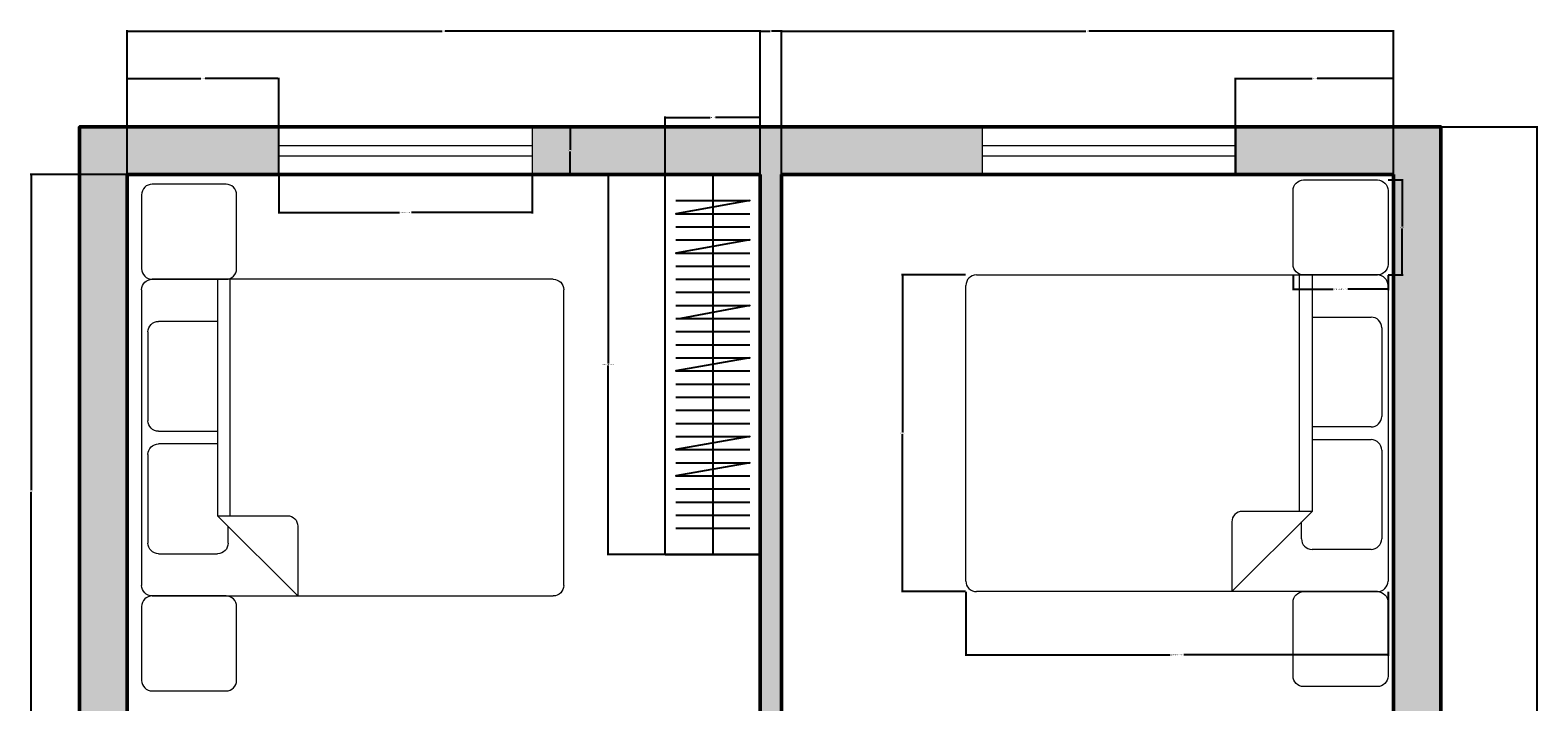
# Model space of a CAD drawing. Units: inches. Extents: x 2130 to 2425, y 2862 to 3216.
# Tile 4 of 4: x 2139 to 2425, y 3089 to 3216. Entities that reach past the tile are written whole.
import ezdxf

# ---------------------------------------------------------------- set-up
doc = ezdxf.new("R2010")
doc.units = ezdxf.units.IN
for name, color, linetype, lineweight in [('A-ANNO-DIMS', 2, 'Continuous', 18), ('A-FLOR-CASE', 9, 'Continuous', 25), ('A-FURN', 8, 'Continuous', 18), ('A-GLAZ', 4, 'Continuous', 18), ('A-WALL', 7, 'Continuous', 50), ('A-WALL-PATT', 18, 'Continuous', 13)]:
    doc.layers.add(name, color=color, linetype=linetype, lineweight=lineweight)
doc.styles.get("Standard").update_dxf_attribs({"font": 'arial.ttf'})
doc.dimstyles.get("Standard").update_dxf_attribs({"dimtxt": 0.18, "dimasz": 0.18, "dimexe": 0.18, "dimexo": 0.0625, "dimgap": 0.09, "dimtad": 0, "dimtih": 1, "dimtoh": 1, "dimdec": 4, "dimzin": 0, "dimdsep": 46, "dimtxsty": 'Standard', "dimcen": 0.09, "dimadec": 0, "dimazin": 0, "dimtfac": 1, "dimtdec": 4, "dimtofl": 0, "dimtmove": 0, "dimatfit": 3, "dimfxl": 1, "dimtolj": 1, "dimtzin": 0, "dimarcsym": 0})

# ---------------------------------------------------------------- blocks, each defined once
blk = doc.blocks.new('Bed - Queen')
for p, q in [((2, 0), (57.99999, 0)), ((0, -78.00003), (0, -2)), ((9.99999, -1.2), (26.79998, -1.2)), ((33.19999, -1.2), (49.99999, -1.2)), ((59.99999, -2), (59.99999, -78.00003)), ((7.99999, -14.4), (7.99999, -3.2)), ((28.79998, -3.2), (28.79998, -14.4)), ((31.19999, -14.4), (31.19999, -3.2)), ((51.99999, -3.2), (51.99999, -14.4)), ((0, -14.4), (44.8, -14.4)), ((44.8, -16.8), (0, -16.8)), ((59.99999, -29.6), (44.8, -14.4)), ((44.8, -14.4), (44.8, -27.6)), ((49.99999, -16.4), (46.79936, -16.4)), ((46.8, -29.6), (59.99999, -29.6)), ((57.99999, -80.00003), (2, -80.00003))]:
    blk.add_line(p, q)
for centre, start, end in [((2, -2), 90, 180), ((57.99999, -2), 0, 90), ((9.99999, -3.2), 90, 180), ((26.79998, -3.2), 0, 90), ((33.19999, -3.2), 90, 180), ((49.99999, -3.2), 0, 90), ((49.99999, -14.4), 270, 0), ((46.8, -27.6), 180, 270), ((2, -78.00003), 180, 270), ((57.99999, -78.00003), 270, 0)]:
    blk.add_arc(centre, 2, start, end)
blk = doc.blocks.new('WIN-48IN')
for p, q in [((0, 0), (0, 9)), ((48, 9), (48, 0)), ((0, 5.5), (48, 5.5)), ((0, 3.5), (48, 3.5))]:
    blk.add_line(p, q)
blk = doc.blocks.new('WARDROBE-72X18IN')
for p, q in [((0, 0), (0, 72)), ((0, 72), (18, 72)), ((9, 72), (9, 0)), ((18, 72), (18, 0)), ((2, 62.07), (16, 62.07)), ((2, 54.62), (16, 54.62)), ((2, 52.14), (16, 52.14)), ((2, 49.66), (16, 49.66)), ((2, 44.69), (16, 44.69)), ((2, 42.21), (16, 42.21)), ((2, 39.72), (16, 39.72)), ((2, 32.28), (16, 32.28)), ((2, 29.79), (16, 29.79)), ((2, 27.31), (16, 27.31)), ((2, 24.83), (16, 24.83)), ((2, 12.41), (16, 12.41)), ((2, 9.93), (16, 9.93)), ((2, 7.45), (16, 7.45)), ((2, 4.97), (16, 4.97)), ((18, 0), (0, 0))]:
    blk.add_line(p, q)
for points in [[(2, 67.03), (16, 67.03), (2, 64.55), (16, 64.55)], [(2, 59.59), (16, 59.59), (2, 57.1), (16, 57.1)], [(2, 47.17), (16, 47.17), (2.98, 44.69)], [(2, 37.24), (16, 37.24), (2, 34.76), (16, 34.76)], [(2, 22.35), (16, 22.35), (2, 19.86), (16, 19.86)], [(2, 17.38), (16, 17.38), (2, 14.9), (16, 14.9)]]:
    blk.add_lwpolyline(points)
blk.add_lwpolyline([(0, 0), (18, 0)], close=True)
blk = doc.blocks.new('NIGHTSTAND-18IN')
blk.add_lwpolyline([(16, 0), (2, 0, -0.414214), (0, 2), (0, 16, -0.414214), (2, 18), (16, 18, -0.414214), (18, 16), (18, 2, -0.414214)], format="xyb", close=True)
blk = doc.blocks.new('*D15')
at = {"layer": 'A-ANNO-DIMS', "color": 0, "lineweight": -2, "transparency": 16777216}
for p, q in [((2186.32, 3188.89), (2186.32, 3181.57)), ((2234.32, 3188.89), (2234.32, 3181.57)), ((2186.5, 3181.75), (2209.2, 3181.75)), ((2234.14, 3181.75), (2211.44, 3181.75))]:
    blk.add_line(p, q, dxfattribs=at)
at = {"layer": 'A-ANNO-DIMS', "color": 0, "transparency": 16777216}
for points in [[(2186.5, 3181.78), (2186.5, 3181.72), (2186.32, 3181.75)], [(2234.14, 3181.78), (2234.14, 3181.72), (2234.32, 3181.75)]]:
    blk.add_solid(points, dxfattribs=at)
at = {"layer": 'Defpoints', "color": 0, "transparency": 16777216}
for p in [(2186.32, 3188.95), (2234.32, 3188.95), (2234.32, 3181.75)]:
    blk.add_point(p, dxfattribs=at)
at = {"layer": 'A-ANNO-DIMS', "color": 0, "transparency": 16777216, "insert": (2210.32, 3181.75), "char_height": 0.18, "attachment_point": 5}
blk.add_mtext('\\A1;WINDOW 48 TYP.', dxfattribs=at)
blk = doc.blocks.new('*D16')
at = {"layer": 'A-ANNO-DIMS', "color": 0, "lineweight": -2, "transparency": 16777216}
for p, q in [((2234.39, 3197.95), (2241.7, 3197.95)), ((2241.52, 3197.77), (2241.52, 3193.64)), ((2241.52, 3189.13), (2241.52, 3193.27)), ((2234.39, 3188.95), (2241.7, 3188.95))]:
    blk.add_line(p, q, dxfattribs=at)
at = {"layer": 'A-ANNO-DIMS', "color": 0, "transparency": 16777216}
for points in [[(2241.49, 3197.77), (2241.55, 3197.77), (2241.52, 3197.95)], [(2241.49, 3189.13), (2241.55, 3189.13), (2241.52, 3188.95)]]:
    blk.add_solid(points, dxfattribs=at)
at = {"layer": 'Defpoints', "color": 0, "transparency": 16777216}
for p in [(2234.32, 3197.95), (2241.52, 3197.95), (2234.32, 3188.95)]:
    blk.add_point(p, dxfattribs=at)
at = {"layer": 'A-ANNO-DIMS', "color": 0, "transparency": 16777216, "insert": (2241.52, 3193.45), "char_height": 0.18, "attachment_point": 5}
blk.add_mtext('\\A1;9 TYP.', dxfattribs=at)
blk = doc.blocks.new('*D17')
at = {"layer": 'A-ANNO-DIMS', "color": 0, "lineweight": -2, "transparency": 16777216}
for p, q in [((2378.51, 3169.85), (2378.51, 3167.03)), ((2396.51, 3169.85), (2396.51, 3167.03)), ((2378.69, 3167.21), (2386.13, 3167.21)), ((2396.33, 3167.21), (2388.89, 3167.21))]:
    blk.add_line(p, q, dxfattribs=at)
at = {"layer": 'A-ANNO-DIMS', "color": 0, "transparency": 16777216}
for points in [[(2378.69, 3167.24), (2378.69, 3167.18), (2378.51, 3167.21)], [(2396.33, 3167.24), (2396.33, 3167.18), (2396.51, 3167.21)]]:
    blk.add_solid(points, dxfattribs=at)
at = {"layer": 'Defpoints', "color": 0, "transparency": 16777216}
for p in [(2378.51, 3169.91), (2396.51, 3169.91), (2396.51, 3167.21)]:
    blk.add_point(p, dxfattribs=at)
at = {"layer": 'A-ANNO-DIMS', "color": 0, "transparency": 16777216, "insert": (2387.51, 3167.21), "char_height": 0.18, "attachment_point": 5}
blk.add_mtext('\\A1;NIGHTSTAND 18 TYP.', dxfattribs=at)
blk = doc.blocks.new('*D18')
at = {"layer": 'A-ANNO-DIMS', "color": 0, "lineweight": -2, "transparency": 16777216}
for p, q in [((2396.57, 3187.91), (2399.39, 3187.91)), ((2399.21, 3187.73), (2399.21, 3179.09)), ((2399.21, 3170.09), (2399.21, 3178.73)), ((2396.57, 3169.91), (2399.39, 3169.91))]:
    blk.add_line(p, q, dxfattribs=at)
at = {"layer": 'A-ANNO-DIMS', "color": 0, "transparency": 16777216}
for points in [[(2399.18, 3187.73), (2399.24, 3187.73), (2399.21, 3187.91)], [(2399.18, 3170.09), (2399.24, 3170.09), (2399.21, 3169.91)]]:
    blk.add_solid(points, dxfattribs=at)
at = {"layer": 'Defpoints', "color": 0, "transparency": 16777216}
for p in [(2396.51, 3187.91), (2399.21, 3187.91), (2396.51, 3169.91)]:
    blk.add_point(p, dxfattribs=at)
at = {"layer": 'A-ANNO-DIMS', "color": 0, "transparency": 16777216, "insert": (2399.21, 3178.91), "char_height": 0.18, "attachment_point": 5}
blk.add_mtext('\\A1;18 TYP.', dxfattribs=at)
blk = doc.blocks.new('*D19')
at = {"layer": 'A-ANNO-DIMS', "color": 0, "lineweight": -2, "transparency": 16777216}
for p, q in [((2259.49, 3188.95), (2248.57, 3188.95)), ((2248.75, 3188.77), (2248.75, 3153.14)), ((2248.75, 3117.13), (2248.75, 3152.77)), ((2259.49, 3116.95), (2248.57, 3116.95))]:
    blk.add_line(p, q, dxfattribs=at)
at = {"layer": 'A-ANNO-DIMS', "color": 0, "transparency": 16777216}
for points in [[(2248.72, 3188.77), (2248.78, 3188.77), (2248.75, 3188.95)], [(2248.72, 3117.13), (2248.78, 3117.13), (2248.75, 3116.95)]]:
    blk.add_solid(points, dxfattribs=at)
at = {"layer": 'Defpoints', "color": 0, "transparency": 16777216}
for p in [(2248.75, 3188.95), (2259.55, 3188.95), (2259.55, 3116.95)]:
    blk.add_point(p, dxfattribs=at)
at = {"layer": 'A-ANNO-DIMS', "color": 0, "transparency": 16777216, "insert": (2248.75, 3152.95), "char_height": 0.18, "attachment_point": 5}
blk.add_mtext('\\A1;WARDROBE 72 TYP.', dxfattribs=at)
blk = doc.blocks.new('*D20')
at = {"layer": 'A-ANNO-DIMS', "color": 0, "lineweight": -2, "transparency": 16777216}
for p, q in [((2259.55, 3189.02), (2259.55, 3199.93)), ((2259.73, 3199.75), (2268.03, 3199.75)), ((2277.37, 3199.75), (2269.07, 3199.75)), ((2277.55, 3189.02), (2277.55, 3199.93))]:
    blk.add_line(p, q, dxfattribs=at)
at = {"layer": 'A-ANNO-DIMS', "color": 0, "transparency": 16777216}
for points in [[(2259.73, 3199.78), (2259.73, 3199.72), (2259.55, 3199.75)], [(2277.37, 3199.78), (2277.37, 3199.72), (2277.55, 3199.75)]]:
    blk.add_solid(points, dxfattribs=at)
at = {"layer": 'Defpoints', "color": 0, "transparency": 16777216}
for p in [(2277.55, 3199.75), (2259.55, 3188.95), (2277.55, 3188.95)]:
    blk.add_point(p, dxfattribs=at)
at = {"layer": 'A-ANNO-DIMS', "color": 0, "transparency": 16777216, "insert": (2268.55, 3199.75), "char_height": 0.18, "attachment_point": 5}
blk.add_mtext('\\A1;18 TYP.', dxfattribs=at)
blk = doc.blocks.new('*D27')
at = {"layer": 'A-ANNO-DIMS', "color": 0, "lineweight": -2, "transparency": 16777216}
for p, q in [((2316.51, 3109.85), (2316.51, 3097.73)), ((2396.51, 3109.85), (2396.51, 3097.73)), ((2316.69, 3097.91), (2355.21, 3097.91)), ((2396.33, 3097.91), (2357.81, 3097.91))]:
    blk.add_line(p, q, dxfattribs=at)
at = {"layer": 'A-ANNO-DIMS', "color": 0, "transparency": 16777216}
for points in [[(2316.69, 3097.94), (2316.69, 3097.88), (2316.51, 3097.91)], [(2396.33, 3097.94), (2396.33, 3097.88), (2396.51, 3097.91)]]:
    blk.add_solid(points, dxfattribs=at)
at = {"layer": 'Defpoints', "color": 0, "transparency": 16777216}
for p in [(2316.51, 3109.91), (2396.51, 3109.91), (2396.51, 3097.91)]:
    blk.add_point(p, dxfattribs=at)
at = {"layer": 'A-ANNO-DIMS', "color": 0, "transparency": 16777216, "insert": (2356.51, 3097.91), "char_height": 0.18, "attachment_point": 5}
blk.add_mtext('\\A1;QUEEN BED 80 TYP.', dxfattribs=at)
blk = doc.blocks.new('*D28')
at = {"layer": 'A-ANNO-DIMS', "color": 0, "lineweight": -2, "transparency": 16777216}
for p, q in [((2316.45, 3169.91), (2304.33, 3169.91)), ((2304.51, 3169.73), (2304.51, 3140.09)), ((2304.51, 3110.09), (2304.51, 3139.73)), ((2316.45, 3109.91), (2304.33, 3109.91))]:
    blk.add_line(p, q, dxfattribs=at)
at = {"layer": 'A-ANNO-DIMS', "color": 0, "transparency": 16777216}
for points in [[(2304.48, 3169.73), (2304.54, 3169.73), (2304.51, 3169.91)], [(2304.48, 3110.09), (2304.54, 3110.09), (2304.51, 3109.91)]]:
    blk.add_solid(points, dxfattribs=at)
at = {"layer": 'Defpoints', "color": 0, "transparency": 16777216}
for p in [(2316.51, 3169.91), (2304.51, 3109.91), (2316.51, 3109.91)]:
    blk.add_point(p, dxfattribs=at)
at = {"layer": 'A-ANNO-DIMS', "color": 0, "transparency": 16777216, "insert": (2304.51, 3139.91), "char_height": 0.18, "attachment_point": 5}
blk.add_mtext('\\A1;60 TYP.', dxfattribs=at)
blk = doc.blocks.new('*D36')
at = {"layer": 'A-ANNO-DIMS', "color": 0, "lineweight": -2, "transparency": 16777216}
for p, q in [((2406.61, 3197.95), (2424.88, 3197.95)), ((2424.7, 3197.77), (2424.7, 3039.14)), ((2424.7, 2880.13), (2424.7, 3038.77)), ((2406.61, 2879.95), (2424.88, 2879.95))]:
    blk.add_line(p, q, dxfattribs=at)
at = {"layer": 'A-ANNO-DIMS', "color": 0, "transparency": 16777216}
for points in [[(2424.67, 3197.77), (2424.73, 3197.77), (2424.7, 3197.95)], [(2424.67, 2880.13), (2424.73, 2880.13), (2424.7, 2879.95)]]:
    blk.add_solid(points, dxfattribs=at)
at = {"layer": 'Defpoints', "color": 0, "transparency": 16777216}
for p in [(2406.55, 3197.95), (2424.7, 3197.95), (2406.55, 2879.95)]:
    blk.add_point(p, dxfattribs=at)
at = {"layer": 'A-ANNO-DIMS', "color": 0, "transparency": 16777216, "insert": (2424.7, 3038.95), "char_height": 0.18, "attachment_point": 5}
blk.add_mtext('\\A1;318', dxfattribs=at)
blk = doc.blocks.new('*D37')
at = {"layer": 'A-ANNO-DIMS', "color": 0, "lineweight": -2, "transparency": 16777216}
for p, q in [((2157.55, 3189.02), (2157.55, 3207.28)), ((2157.73, 3207.1), (2171.54, 3207.1)), ((2186.14, 3207.1), (2172.33, 3207.1)), ((2186.32, 3189.02), (2186.32, 3207.28))]:
    blk.add_line(p, q, dxfattribs=at)
at = {"layer": 'A-ANNO-DIMS', "color": 0, "transparency": 16777216}
for points in [[(2157.73, 3207.13), (2157.73, 3207.07), (2157.55, 3207.1)], [(2186.14, 3207.13), (2186.14, 3207.07), (2186.32, 3207.1)]]:
    blk.add_solid(points, dxfattribs=at)
at = {"layer": 'Defpoints', "color": 0, "transparency": 16777216}
for p in [(2186.32, 3207.1), (2157.55, 3188.95), (2186.32, 3188.95)]:
    blk.add_point(p, dxfattribs=at)
at = {"layer": 'A-ANNO-DIMS', "color": 0, "transparency": 16777216, "insert": (2171.94, 3207.1), "char_height": 0.18, "attachment_point": 5}
blk.add_mtext('\\A1;28.77', dxfattribs=at)
blk = doc.blocks.new('*D38')
at = {"layer": 'A-ANNO-DIMS', "color": 0, "lineweight": -2, "transparency": 16777216}
for p, q in [((2367.64, 3189.02), (2367.64, 3207.28)), ((2367.82, 3207.1), (2382.13, 3207.1)), ((2397.37, 3207.1), (2383.06, 3207.1)), ((2397.55, 3189.02), (2397.55, 3207.28))]:
    blk.add_line(p, q, dxfattribs=at)
at = {"layer": 'A-ANNO-DIMS', "color": 0, "transparency": 16777216}
for points in [[(2367.82, 3207.13), (2367.82, 3207.07), (2367.64, 3207.1)], [(2397.37, 3207.13), (2397.37, 3207.07), (2397.55, 3207.1)]]:
    blk.add_solid(points, dxfattribs=at)
at = {"layer": 'Defpoints', "color": 0, "transparency": 16777216}
for p in [(2397.55, 3207.1), (2367.64, 3188.95), (2397.55, 3188.95)]:
    blk.add_point(p, dxfattribs=at)
at = {"layer": 'A-ANNO-DIMS', "color": 0, "transparency": 16777216, "insert": (2382.6, 3207.1), "char_height": 0.18, "attachment_point": 5}
blk.add_mtext('\\A1;29.907', dxfattribs=at)
blk = doc.blocks.new('*D46')
at = {"layer": 'A-ANNO-DIMS', "color": 0, "lineweight": -2, "transparency": 16777216}
for p, q in [((2157.55, 3189.02), (2157.55, 3216.28)), ((2157.73, 3216.1), (2217.27, 3216.1)), ((2277.37, 3216.1), (2217.83, 3216.1)), ((2277.55, 3189.02), (2277.55, 3216.28))]:
    blk.add_line(p, q, dxfattribs=at)
at = {"layer": 'A-ANNO-DIMS', "color": 0, "transparency": 16777216}
for points in [[(2157.73, 3216.13), (2157.73, 3216.07), (2157.55, 3216.1)], [(2277.37, 3216.13), (2277.37, 3216.07), (2277.55, 3216.1)]]:
    blk.add_solid(points, dxfattribs=at)
at = {"layer": 'Defpoints', "color": 0, "transparency": 16777216}
for p in [(2277.55, 3216.1), (2157.55, 3188.95), (2277.55, 3188.95)]:
    blk.add_point(p, dxfattribs=at)
at = {"layer": 'A-ANNO-DIMS', "color": 0, "transparency": 16777216, "insert": (2217.55, 3216.1), "char_height": 0.18, "attachment_point": 5}
blk.add_mtext('\\A1;120', dxfattribs=at)
blk = doc.blocks.new('*D47')
at = {"layer": 'A-ANNO-DIMS', "color": 0, "lineweight": -2, "transparency": 16777216}
for p, q in [((2277.55, 3189.02), (2277.55, 3216.28)), ((2277.73, 3216.1), (2279.4, 3216.1)), ((2281.37, 3216.1), (2279.7, 3216.1)), ((2281.55, 3189.02), (2281.55, 3216.28))]:
    blk.add_line(p, q, dxfattribs=at)
at = {"layer": 'A-ANNO-DIMS', "color": 0, "transparency": 16777216}
for points in [[(2277.73, 3216.13), (2277.73, 3216.07), (2277.55, 3216.1)], [(2281.37, 3216.13), (2281.37, 3216.07), (2281.55, 3216.1)]]:
    blk.add_solid(points, dxfattribs=at)
at = {"layer": 'Defpoints', "color": 0, "transparency": 16777216}
for p in [(2281.55, 3216.1), (2277.55, 3188.95), (2281.55, 3188.95)]:
    blk.add_point(p, dxfattribs=at)
at = {"layer": 'A-ANNO-DIMS', "color": 0, "transparency": 16777216, "insert": (2279.55, 3216.1), "char_height": 0.18, "attachment_point": 5}
blk.add_mtext('\\A1;4', dxfattribs=at)
blk = doc.blocks.new('*D48')
at = {"layer": 'A-ANNO-DIMS', "color": 0, "lineweight": -2, "transparency": 16777216}
for p, q in [((2281.55, 3189.02), (2281.55, 3216.28)), ((2281.73, 3216.1), (2339.27, 3216.1)), ((2397.37, 3216.1), (2339.83, 3216.1)), ((2397.55, 3189.02), (2397.55, 3216.28))]:
    blk.add_line(p, q, dxfattribs=at)
at = {"layer": 'A-ANNO-DIMS', "color": 0, "transparency": 16777216}
for points in [[(2281.73, 3216.13), (2281.73, 3216.07), (2281.55, 3216.1)], [(2397.37, 3216.13), (2397.37, 3216.07), (2397.55, 3216.1)]]:
    blk.add_solid(points, dxfattribs=at)
at = {"layer": 'Defpoints', "color": 0, "transparency": 16777216}
for p in [(2397.55, 3216.1), (2281.55, 3188.95), (2397.55, 3188.95)]:
    blk.add_point(p, dxfattribs=at)
at = {"layer": 'A-ANNO-DIMS', "color": 0, "transparency": 16777216, "insert": (2339.55, 3216.1), "char_height": 0.18, "attachment_point": 5}
blk.add_mtext('\\A1;116', dxfattribs=at)
blk = doc.blocks.new('*D49')
at = {"layer": 'A-ANNO-DIMS', "color": 0, "lineweight": -2, "transparency": 16777216}
for p, q in [((2157.49, 3188.95), (2139.22, 3188.95)), ((2139.4, 3188.77), (2139.4, 3129.14)), ((2139.4, 3069.13), (2139.4, 3128.77)), ((2157.49, 3068.95), (2139.22, 3068.95))]:
    blk.add_line(p, q, dxfattribs=at)
at = {"layer": 'A-ANNO-DIMS', "color": 0, "transparency": 16777216}
for points in [[(2139.37, 3188.77), (2139.43, 3188.77), (2139.4, 3188.95)], [(2139.37, 3069.13), (2139.43, 3069.13), (2139.4, 3068.95)]]:
    blk.add_solid(points, dxfattribs=at)
at = {"layer": 'Defpoints', "color": 0, "transparency": 16777216}
for p in [(2139.4, 3188.95), (2157.55, 3188.95), (2157.55, 3068.95)]:
    blk.add_point(p, dxfattribs=at)
at = {"layer": 'A-ANNO-DIMS', "color": 0, "transparency": 16777216, "insert": (2139.4, 3128.95), "char_height": 0.18, "attachment_point": 5}
blk.add_mtext('\\A1;120', dxfattribs=at)

msp = doc.modelspace()

# ---------------------------------------------------------------- hatches: boundary and pattern name
at = {"layer": 'A-WALL-PATT'}
h = msp.add_hatch(color=256, dxfattribs=at)
h.dxf.hatch_style = 1
h.paths.add_polyline_path([(2186.3228, 3197.9544), (2148.5502, 3197.9544), (2148.5502, 3046.791), (2157.5502, 3046.791), (2157.5502, 3064.9544), (2217.5502, 3064.9544), (2217.5502, 3058.9544), (2221.1502, 3058.9544), (2221.5502, 3058.9544), (2221.5502, 3064.9544), (2241.5502, 3064.9544), (2241.5502, 3068.9544), (2157.5502, 3068.9544), (2157.5502, 3086.9544), (2157.5502, 3188.9544), (2186.3228, 3188.9544)])
h = msp.add_hatch(color=256, dxfattribs=at)
h.dxf.hatch_style = 1
h.paths.add_polyline_path([(2319.6433, 3197.9544), (2234.3228, 3197.9544), (2234.3228, 3188.9544), (2277.5502, 3188.9544), (2277.5502, 3116.9544), (2277.5502, 3068.9544), (2271.5502, 3068.9544), (2271.5502, 3064.9544), (2281.5502, 3064.9544), (2287.5502, 3064.9544), (2287.5502, 3068.9544), (2281.5502, 3068.9544), (2281.5502, 3188.9544), (2319.6433, 3188.9544)])
h = msp.add_hatch(color=256, dxfattribs=at)
h.dxf.hatch_style = 1
h.paths.add_polyline_path([(2406.5502, 3197.9544), (2367.6433, 3197.9544), (2367.6433, 3188.9544), (2397.5502, 3188.9544), (2397.5502, 3068.9544), (2325.5502, 3068.9544), (2317.5502, 3068.9544), (2317.5502, 3064.9544), (2323.5502, 3064.9544), (2323.5502, 3056.9544), (2327.5502, 3056.9544), (2327.5502, 3064.9544), (2397.5502, 3064.9544), (2397.5502, 2990.9544), (2327.5502, 2990.9544), (2327.5502, 3032.9544), (2323.5502, 3032.9544), (2323.5502, 2986.9544), (2323.5502, 2961.9544), (2327.5502, 2961.9544), (2327.5502, 2986.9544), (2397.5502, 2986.9544), (2397.5502, 2966.8556), (2406.5502, 2966.8556)])

# ---------------------------------------------------------------- linework, layer by layer
at = {"layer": 'A-WALL'}
for p, q in [((2157.5502, 3188.9544), (2277.5502, 3188.9544)), ((2157.5502, 3068.9544), (2157.5502, 3188.9544)), ((2277.5502, 3068.9544), (2277.5502, 3188.9544)), ((2281.5502, 3188.9544), (2397.5502, 3188.9544)), ((2281.5502, 3068.9544), (2281.5502, 3188.9544)), ((2397.5502, 3188.9544), (2397.5502, 3068.9544))]:
    msp.add_line(p, q, dxfattribs=at)
msp.add_lwpolyline([(2163.5502, 2879.9544), (2148.5502, 2879.9544), (2148.5502, 3197.9544), (2406.5502, 3197.9544), (2406.5502, 2879.9544), (2211.5502, 2879.9544)], dxfattribs=at)

# ---------------------------------------------------------------- block references
at = {"layer": 'A-FLOR-CASE'}
msp.add_blockref('WARDROBE-72X18IN', (2259.55, 3116.954), dxfattribs=at)
at = {"layer": 'A-FURN', "extrusion": (0, 0, -1), "zscale": -1}
for p in [(-2178.3158, 3169.097), (-2178.3158, 3091.097)]:
    msp.add_blockref('NIGHTSTAND-18IN', p, dxfattribs=at)
at = {"layer": 'A-FURN'}
for p in [(2378.511, 3169.909), (2378.511, 3091.909)]:
    msp.add_blockref('NIGHTSTAND-18IN', p, dxfattribs=at)
at = {"layer": 'A-FURN', "xscale": -1, "rotation": 90}
msp.add_blockref('Bed - Queen', (2160.3162, 3169.097), dxfattribs=at)
at = {"layer": 'A-FURN', "rotation": 270}
msp.add_blockref('Bed - Queen', (2396.5106, 3169.909), dxfattribs=at)
at = {"layer": 'A-GLAZ'}
for p in [(2186.323, 3188.954), (2319.6436, 3188.954)]:
    msp.add_blockref('WIN-48IN', p, dxfattribs=at)

# ---------------------------------------------------------------- dimensions: what is measured, and where the dimension line sits
at = {"layer": 'A-ANNO-DIMS'}
for base, p1, p2, override, picture, middle in [((2277.5502, 3216.1044), (2157.5502, 3188.9544), (2277.5502, 3188.9544), {"dimdec": 0, "dimlfac": 1, "dimrnd": 0, "dimzin": 0, "dimdsep": 46, "dimlunit": 2}, '*D46', (2217.5502, 3216.1044)), ((2281.5502, 3216.1044), (2277.5502, 3188.9544), (2281.5502, 3188.9544), {"dimdec": 0, "dimlfac": 1, "dimrnd": 0, "dimzin": 0, "dimdsep": 46, "dimlunit": 2}, '*D47', (2279.5502, 3216.1044)), ((2397.5502, 3216.1044), (2281.5502, 3188.9544), (2397.5502, 3188.9544), {"dimdec": 0, "dimlfac": 1, "dimrnd": 0, "dimzin": 0, "dimdsep": 46, "dimlunit": 2}, '*D48', (2339.5502, 3216.1044)), ((2397.5502, 3207.1044), (2367.6433, 3188.9544), (2397.5502, 3188.9544), {"dimdec": 3, "dimlfac": 1, "dimrnd": 0, "dimzin": 0, "dimdsep": 46, "dimlunit": 2}, '*D38', (2382.5968, 3207.1044))]:
    dim = msp.add_linear_dim(base=base, p1=p1, p2=p2, dimstyle='Standard', override=override, dxfattribs=at)
    dim.commit()
    dim.dimension.update_dxf_attribs({"geometry": picture, "text_midpoint": middle})
for base, p1, p2, angle, override, picture, middle in [((2186.3228, 3207.1044), (2157.5502, 3188.9544), (2186.3228, 3188.9544), 0, {"dimdec": 2, "dimlfac": 1, "dimrnd": 0, "dimzin": 0, "dimdsep": 46, "dimlunit": 2}, '*D37', (2171.9365, 3207.1044)), ((2424.7002, 3197.9544), (2406.5502, 2879.9544), (2406.5502, 3197.9544), 90, {"dimdec": 0, "dimlfac": 1, "dimrnd": 0, "dimzin": 0, "dimdsep": 46, "dimlunit": 2}, '*D36', (2424.7002, 3038.9544)), ((2139.4002, 3188.9544), (2157.5502, 3068.9544), (2157.5502, 3188.9544), 90, {"dimdec": 0, "dimlfac": 1, "dimrnd": 0, "dimzin": 0, "dimdsep": 46, "dimlunit": 2}, '*D49', (2139.4002, 3128.9544))]:
    dim = msp.add_linear_dim(base=base, p1=p1, p2=p2, angle=angle, dimstyle='Standard', override=override, dxfattribs=at)
    dim.commit()
    dim.dimension.update_dxf_attribs({"geometry": picture, "text_midpoint": middle})
for base, p1, p2, text, picture, middle in [((2277.5502, 3199.7544), (2259.5502, 3188.9544), (2277.5502, 3188.9544), '<> TYP.', '*D20', (2268.5502, 3199.7544)), ((2234.3228, 3181.7544), (2186.3228, 3188.9544), (2234.3228, 3188.9544), 'WINDOW <> TYP.', '*D15', (2210.3228, 3181.7544)), ((2396.5106, 3167.209), (2378.5106, 3169.909), (2396.5106, 3169.909), 'NIGHTSTAND <> TYP.', '*D17', (2387.5106, 3167.209)), ((2396.5106, 3097.909), (2316.5106, 3109.909), (2396.5106, 3109.909), 'QUEEN BED <> TYP.', '*D27', (2356.5106, 3097.909))]:
    dim = msp.add_linear_dim(base=base, p1=p1, p2=p2, text=text, dimstyle='Standard', override={"dimdec": 0, "dimlfac": 1, "dimrnd": 0, "dimzin": 0, "dimdsep": 46, "dimlunit": 2}, dxfattribs=at)
    dim.commit()
    dim.dimension.update_dxf_attribs({"geometry": picture, "text_midpoint": middle})
for base, p1, p2, angle, text, picture, middle in [((2241.5228, 3197.9544), (2234.3228, 3188.9544), (2234.3228, 3197.9544), 90, '<> TYP.', '*D16', (2241.5228, 3193.4544)), ((2248.7502, 3188.9544), (2259.5502, 3116.9544), (2259.5502, 3188.9544), 90, 'WARDROBE <> TYP.', '*D19', (2248.7502, 3152.9544)), ((2399.2106, 3187.909), (2396.5106, 3169.909), (2396.5106, 3187.909), 90, '<> TYP.', '*D18', (2399.2106, 3178.909)), ((2304.5106, 3109.909), (2316.5106, 3169.909), (2316.5106, 3109.909), 270, '<> TYP.', '*D28', (2304.5106, 3139.909))]:
    dim = msp.add_linear_dim(base=base, p1=p1, p2=p2, angle=angle, text=text, dimstyle='Standard', override={"dimdec": 0, "dimlfac": 1, "dimrnd": 0, "dimzin": 0, "dimdsep": 46, "dimlunit": 2}, dxfattribs=at)
    dim.commit()
    dim.dimension.update_dxf_attribs({"geometry": picture, "text_midpoint": middle})

doc.saveas('drawing.dxf')
